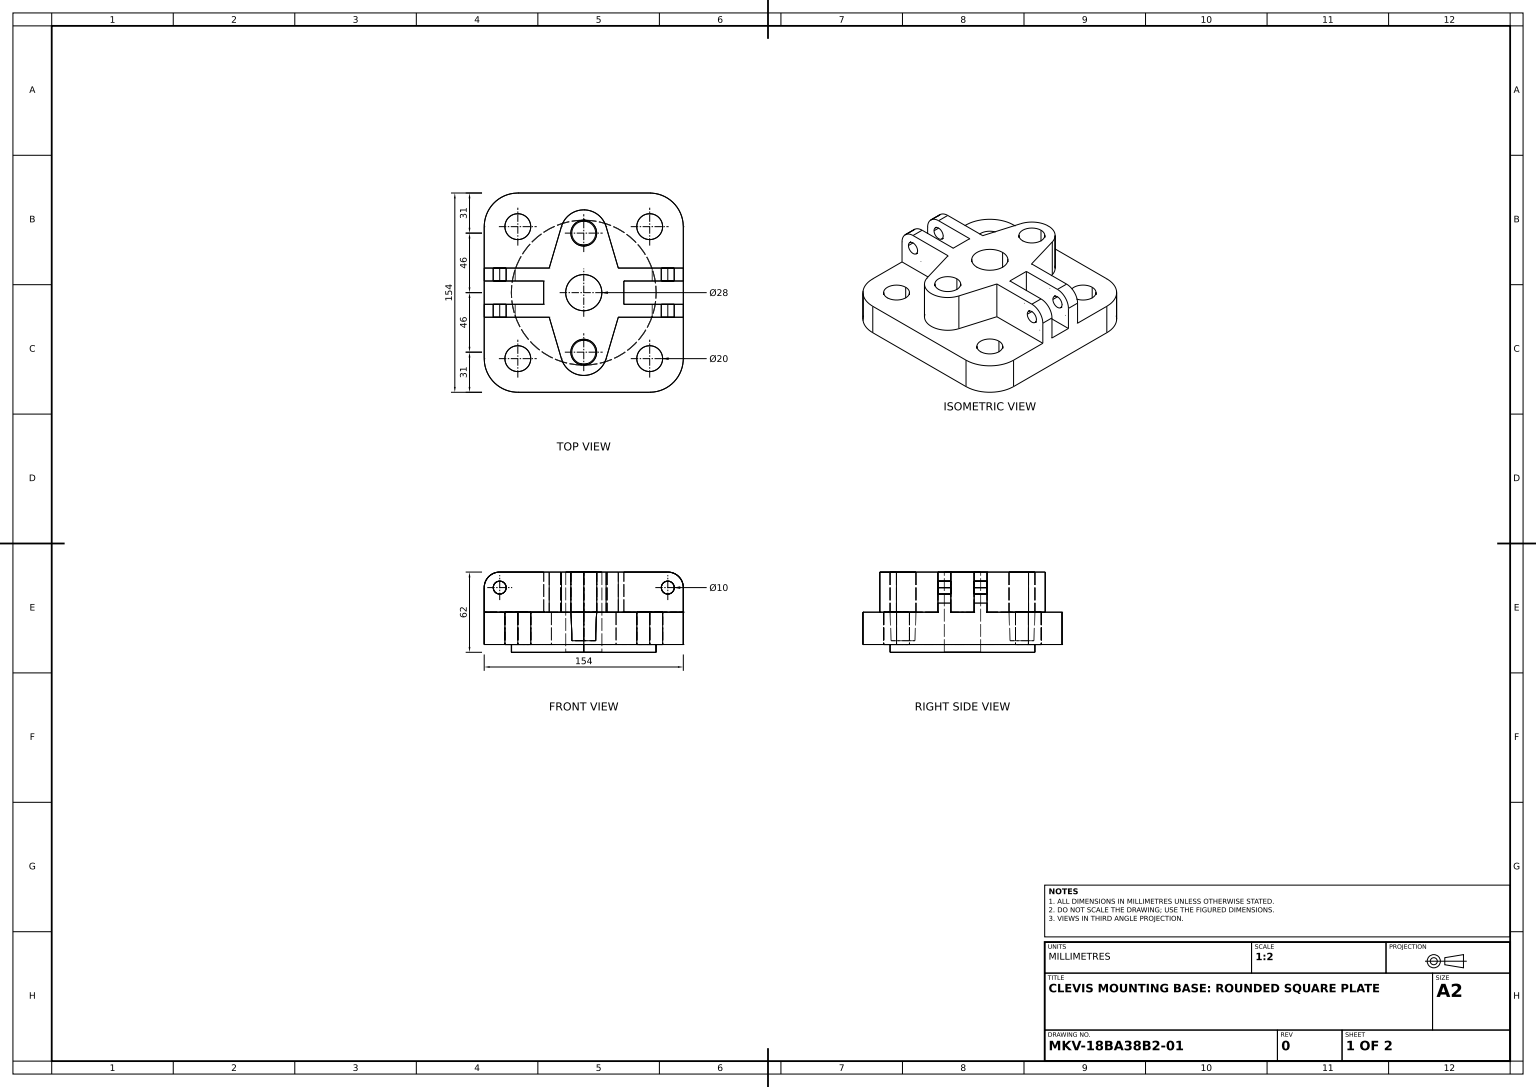
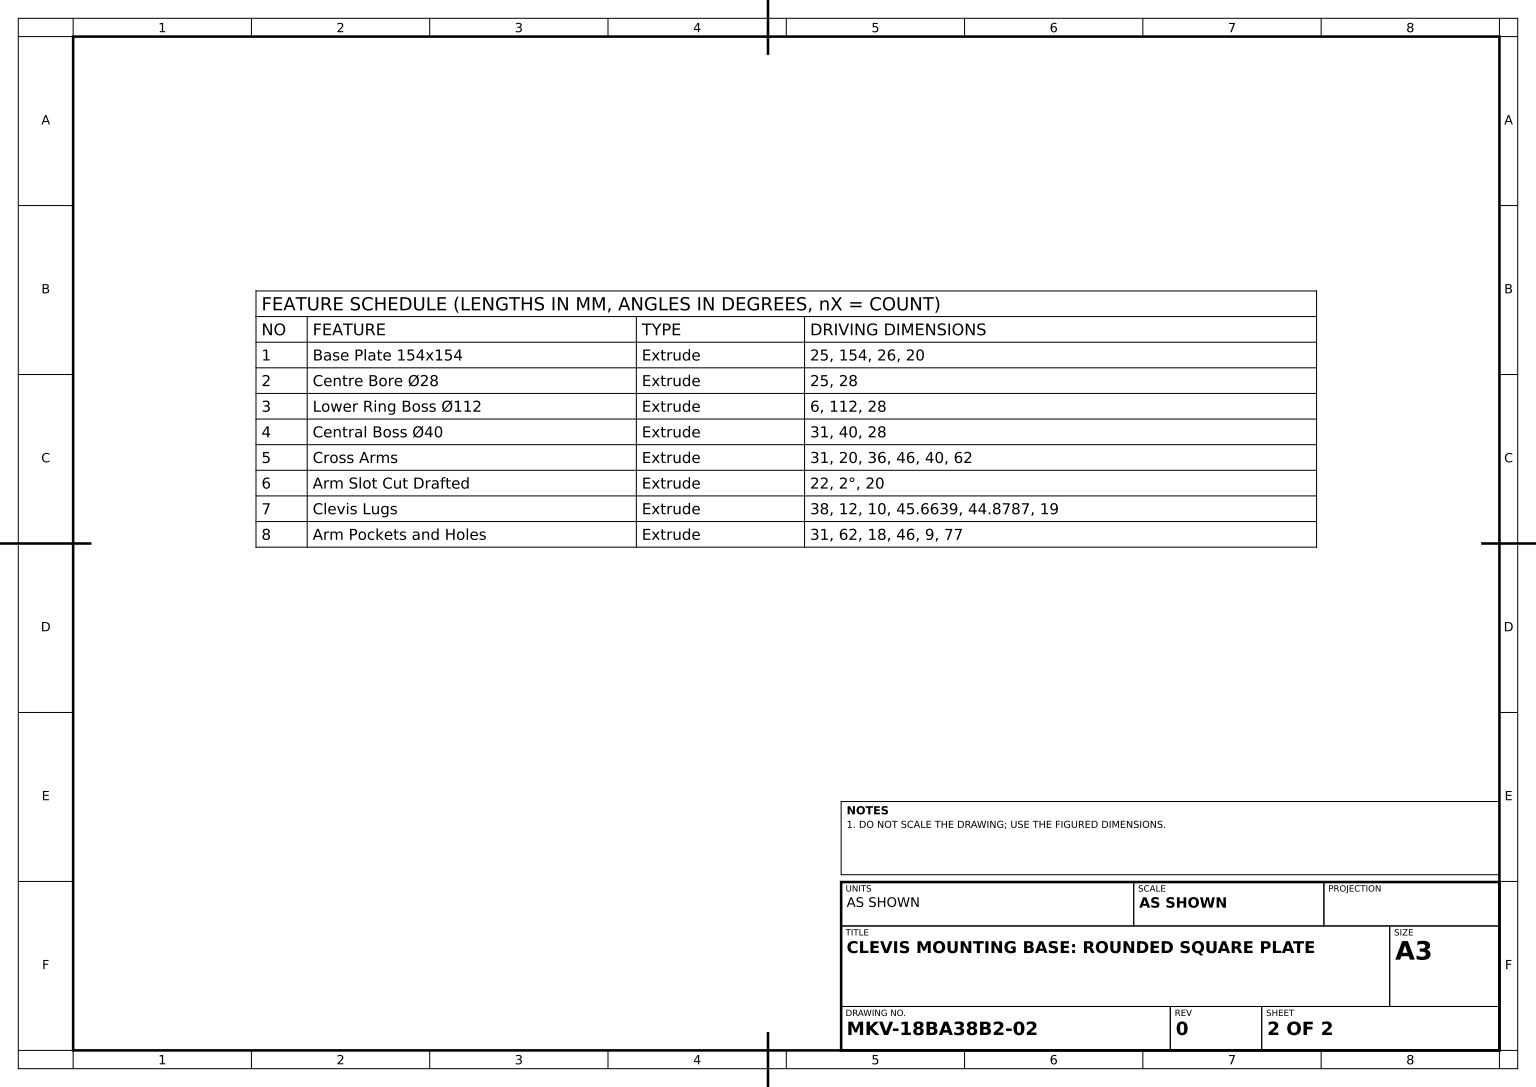
from build123d import *

# Parameters (mm, degrees)
BASE_PLATE_SKETCH_R                  = 10
BASE_PLATE_154X154_DEPTH             = 25
CENTRE_BORE_SKETCH_R                 = 14
CENTRE_BORE_28_DEPTH                 = 25
LOWER_RING_BOSS_SKETCH_R             = 56
LOWER_RING_BOSS_SKETCH_R_2           = 14
LOWER_RING_BOSS_112_DEPTH            = 6
CENTRAL_START                        = 31
CENTRAL_BOSS_SKETCH_R                = 20
CENTRAL_BOSS_SKETCH_R_2              = 14
CENTRAL_BOSS_40_DEPTH                = 31
CROSS_START                          = 31
CROSS_ARMS_SKETCH_R                  = 10
CROSS_ARMS_SKETCH_R_2                = 20
CROSS_ARMS_DEPTH                     = 31
ARM_SLOT_SKETCH_R                    = 10
ARM_SLOT_CUT_DRAFTED_DEPTH           = 22
ARM_SLOT_CUT_DRAFTED_DRAFT           = -2
ARM_SLOT_CUT_DRAFTED_PROFILE_2_DEPTH = 22
ARM_SLOT_CUT_DRAFTED_PROFILE_2_DRAFT = -2
CLEVIS_LUGS_SKETCH_R                 = 5
CLEVIS_LUGS_DEPTH                    = 19
ARM_POCKETS_SKETCH_W                 = 12
ARM_POCKETS_SKETCH_H                 = 18
ARM_POCKETS_AND_HOLES_DEPTH          = 31


with BuildPart() as part:
    # Base Plate Sketch → Base Plate 154x154 (new body)
    with BuildSketch(Plane(origin=(0, 0, 0), x_dir=(1, 0, 0), z_dir=(0, 1, 0))):
        with BuildLine():
            Line((-51, 77), (51, 77))
            ThreePointArc((51, 77), (69.384776311, 69.384776311), (77, 51))
            Line((77, 51), (77, -51))
            ThreePointArc((77, -51), (69.384776311, -69.384776311), (51, -77))
            Line((51, -77), (-51, -77))
            ThreePointArc((-51, -77), (-69.384776311, -69.384776311), (-77, -51))
            Line((-77, -51), (-77, 51))
            ThreePointArc((-77, 51), (-69.384776311, 69.384776311), (-51, 77))
        make_face()
        with Locations(Location((-51, 51, 0), (0, 0, 270))):
            Circle(BASE_PLATE_SKETCH_R, mode=Mode.SUBTRACT)
        with Locations(Location((51, 51, 0), (0, 0, 270))):
            Circle(BASE_PLATE_SKETCH_R, mode=Mode.SUBTRACT)
        with Locations(Location((51, -51, 0), (0, 0, 270))):
            Circle(BASE_PLATE_SKETCH_R, mode=Mode.SUBTRACT)
        with Locations(Location((-51, -51, 0), (0, 0, 270))):
            Circle(BASE_PLATE_SKETCH_R, mode=Mode.SUBTRACT)
    extrude(amount=BASE_PLATE_154X154_DEPTH)

    # Centre Bore Sketch → Centre Bore Ø28 (cut)
    with BuildSketch(Plane(origin=(0, 25, 0), x_dir=(1, 0, 0), z_dir=(0, 1, 0))):
        with Locations(Location((0, 0, 0), (0, 0, 270))):
            Circle(CENTRE_BORE_SKETCH_R)
    extrude(amount=-CENTRE_BORE_28_DEPTH, mode=Mode.SUBTRACT)

    # Lower Ring Boss Sketch → Lower Ring Boss Ø112 (add)
    with BuildSketch(Plane.XZ):
        with Locations(Location((0, 0, 0), (0, 0, 270))):
            Circle(LOWER_RING_BOSS_SKETCH_R)
        with Locations(Location((0, 0, 0), (0, 0, 90))):
            Circle(LOWER_RING_BOSS_SKETCH_R_2, mode=Mode.SUBTRACT)
    extrude(amount=LOWER_RING_BOSS_112_DEPTH)

    # Central Boss Sketch → Central Boss Ø40 (add)
    with BuildSketch(Plane(origin=(0, 25, 0), x_dir=(1, 0, 0), z_dir=(0, 1, 0)).offset(CENTRAL_START)):
        with Locations(Location((0, 0, 0), (0, 0, 270))):
            Circle(CENTRAL_BOSS_SKETCH_R)
        with Locations(Location((0, 0, 0), (0, 0, 270))):
            Circle(CENTRAL_BOSS_SKETCH_R_2, mode=Mode.SUBTRACT)
    extrude(amount=-CENTRAL_BOSS_40_DEPTH)

    # Cross Arms Sketch → Cross Arms (add)
    with BuildSketch(Plane(origin=(0, 25, 0), x_dir=(1, 0, 0), z_dir=(0, 1, 0)).offset(CROSS_START)):
        with BuildLine():
            Line((-29.736293724, 8.760869565), (-17.266235066, 51.086956522))
            ThreePointArc((-17.266235066, 51.086956522), (0, 64), (17.266235066, 51.086956522))
            Line((17.266235066, 51.086956522), (29.736293724, 8.760869565))
            ThreePointArc((29.736293724, 8.760869565), (31, 0), (29.736293724, -8.760869565))
            Line((29.736293724, -8.760869565), (17.266235066, -51.086956522))
            ThreePointArc((17.266235066, -51.086956522), (0, -64), (-17.266235066, -51.086956522))
            Line((-17.266235066, -51.086956522), (-29.736293724, -8.760869565))
            ThreePointArc((-29.736293724, -8.760869565), (-31, 0), (-29.736293724, 8.760869565))
        make_face()
        with Locations(Location((0, 46, 0), (0, 0, 270))):
            Circle(CROSS_ARMS_SKETCH_R, mode=Mode.SUBTRACT)
        with Locations(Location((0, -46, 0), (0, 0, 270))):
            Circle(CROSS_ARMS_SKETCH_R, mode=Mode.SUBTRACT)
        Circle(CROSS_ARMS_SKETCH_R_2, mode=Mode.SUBTRACT)
    extrude(amount=-CROSS_ARMS_DEPTH)


with BuildPart() as arm_slot_cut_drafted_tool:
    # Arm Slot Sketch → Arm Slot Cut Drafted (with draft: the straight prism first)
    with BuildSketch(Plane(origin=(0, 25, 0), x_dir=(1, 0, 0), z_dir=(0, 1, 0))):
        with Locations(Location((0, 46, 0), (0, 0, 270))):
            Circle(ARM_SLOT_SKETCH_R)
    extrude(amount=-ARM_SLOT_CUT_DRAFTED_DEPTH)
    # Arm Slot Cut Drafted: the draft: its side faces are tilted about the plane it starts from
    arm_slot_cut_drafted_sides = [arm_slot_cut_drafted_tool.faces().sort_by_distance(p)[0] for p in [
        (0, 14, -56),
    ]]
    draft(arm_slot_cut_drafted_sides, Plane(origin=(0, 25, 0), x_dir=(1, 0, 0), z_dir=(0, 1, 0)), ARM_SLOT_CUT_DRAFTED_DRAFT)


with BuildPart() as part_1:
    add(part.part)

    # Arm Slot Cut Drafted: cut by arm_slot_cut_drafted_tool
    add(arm_slot_cut_drafted_tool.part, mode=Mode.SUBTRACT)


with BuildPart() as arm_slot_cut_drafted_profile_2_tool:
    # Arm Slot Sketch → Arm Slot Cut Drafted profile 2 (with draft: the straight prism first)
    with BuildSketch(Plane(origin=(0, 25, 0), x_dir=(1, 0, 0), z_dir=(0, 1, 0))):
        with Locations(Location((0, -46, 0), (0, 0, 270))):
            Circle(ARM_SLOT_SKETCH_R)
    extrude(amount=-ARM_SLOT_CUT_DRAFTED_PROFILE_2_DEPTH)
    # Arm Slot Cut Drafted profile 2: the draft: its side faces are tilted about the plane it starts from
    arm_slot_cut_drafted_profile_2_sides = [arm_slot_cut_drafted_profile_2_tool.faces().sort_by_distance(p)[0] for p in [
        (0, 14, 36),
    ]]
    draft(arm_slot_cut_drafted_profile_2_sides, Plane(origin=(0, 25, 0), x_dir=(1, 0, 0), z_dir=(0, 1, 0)), ARM_SLOT_CUT_DRAFTED_PROFILE_2_DRAFT)


with BuildPart() as part_2:
    add(part_1.part)

    # Arm Slot Cut Drafted profile 2: cut by arm_slot_cut_drafted_profile_2_tool
    add(arm_slot_cut_drafted_profile_2_tool.part, mode=Mode.SUBTRACT)

    # Clevis Lugs Sketch → Clevis Lugs (add, symmetric)
    # profile 1 of 2: a face of its own
    with BuildSketch(Plane.XY):
        with BuildLine():
            Line((-19.336072892, 56), (-65, 56))
            ThreePointArc((-65, 56), (-73.485281374, 52.485281374), (-77, 44))
            Line((-77, 44), (-77, 25))
            Line((-77, 25), (-19.336072892, 25))
            Line((-19.336072892, 25), (-19.336072892, 56))
        make_face()
        with Locations((-65, 44)):
            Circle(CLEVIS_LUGS_SKETCH_R, mode=Mode.SUBTRACT)
    # profile 2 of 2: a face of its own
    with BuildSketch(Plane.XY):
        with BuildLine():
            Line((77, 25), (77, 44))
            ThreePointArc((77, 44), (73.485281374, 52.485281374), (65, 56))
            Line((65, 56), (20.121294127, 56))
            Line((20.121294127, 56), (20.121294127, 25))
            Line((20.121294127, 25), (77, 25))
        make_face()
        with Locations((65, 44)):
            Circle(CLEVIS_LUGS_SKETCH_R, mode=Mode.SUBTRACT)
    extrude(amount=CLEVIS_LUGS_DEPTH, both=True)

    # Arm Pockets Sketch → Arm Pockets and Holes (cut)
    with BuildSketch(Plane(origin=(0, 56, 0), x_dir=(1, 0, 0), z_dir=(0, 1, 0))):
        Polygon((-31, 9), (-65, 9), (-65, -9), (-31, -9), (-31, 0), align=None)
        with Locations((-71, 0)):
            Rectangle(ARM_POCKETS_SKETCH_W, ARM_POCKETS_SKETCH_H)
        Polygon((31, 9), (31, 0), (31, -9), (65, -9), (65, 9), align=None)
        with Locations((71, 0)):
            Rectangle(ARM_POCKETS_SKETCH_W, ARM_POCKETS_SKETCH_H)
    extrude(amount=-ARM_POCKETS_AND_HOLES_DEPTH, mode=Mode.SUBTRACT)


solid = part_2.part
